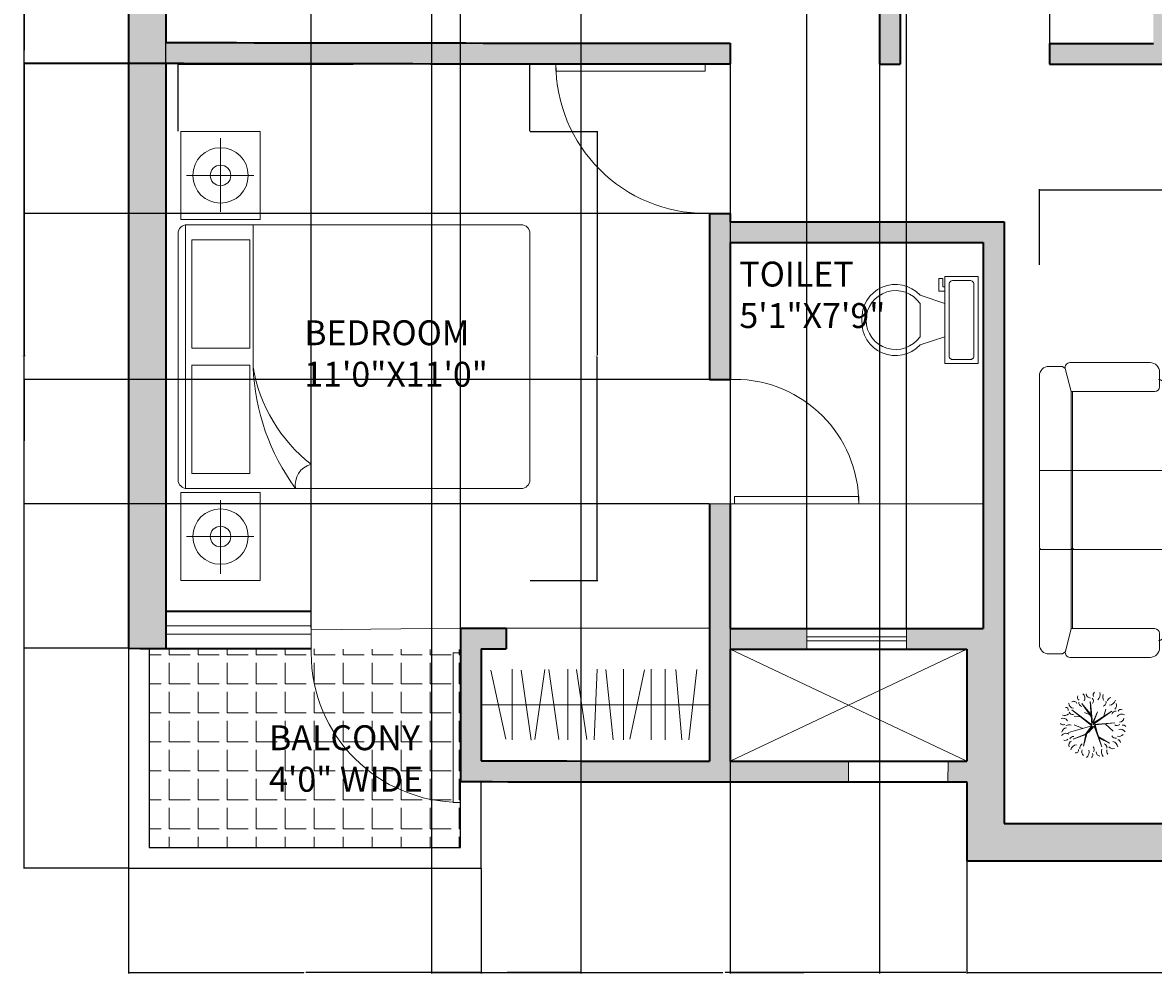
# Model space of a CAD drawing. Units: inches. Extents: x 1044 to 1567, y 918 to 1417.
# Tile 1 of 4: x 1044 to 1316, y 918 to 1148. Entities that reach past the tile are written whole.
import ezdxf

# ---------------------------------------------------------------- set-up
doc = ezdxf.new("R2010")
doc.units = ezdxf.units.IN
for name, color, linetype, lineweight in [('A-ANNO-DIMS', 2, 'Continuous', 18), ('A-AREA-IDEN', 7, 'Continuous', 18), ('A-FLOR', 7, 'Continuous', 13), ('A-FLOR-CASE', 8, 'Continuous', 18), ('A-FLOR-FIXT', 9, 'Continuous', 18), ('A-FLOR-OPEN', 8, 'Continuous', 13), ('A-FLOR-PATT', 9, 'Continuous', 13), ('A-FURN', 8, 'Continuous', 18), ('A-GLAZ', 4, 'Continuous', 13), ('A-WALL', 7, 'Continuous', 35), ('A-WALL-PATT', 252, 'Continuous', 13), ('A-WALL-PRPT', 7, 'Continuous', 25), ('door', 4, 'Continuous', 18)]:
    doc.layers.add(name, color=color, linetype=linetype, lineweight=lineweight)
doc.styles.get("Standard").update_dxf_attribs({"font": 'arial.ttf'})
doc.dimstyles.get("Standard").update_dxf_attribs({"dimtxt": 0.18, "dimasz": 0.18, "dimexe": 0.18, "dimexo": 0.0625, "dimgap": 0.09, "dimtad": 0, "dimtih": 1, "dimtoh": 1, "dimdec": 4, "dimzin": 0, "dimdsep": 46, "dimtxsty": 'Standard', "dimcen": 0.09, "dimadec": 0, "dimazin": 0, "dimtfac": 1, "dimtdec": 4, "dimtofl": 0, "dimtmove": 0, "dimatfit": 3, "dimfxl": 1, "dimtolj": 1, "dimtzin": 0, "dimarcsym": 0})

# ---------------------------------------------------------------- blocks, each defined once
blk = doc.blocks.new('*U4')
for p, q in [((0, 0), (0, 6)), ((36, 0), (36, 6))]:
    blk.add_line(p, q)
blk.add_lwpolyline([(0, 0), (0, -36), (1.75, -36), (1.75, 0)], close=True)
blk.add_arc((0, 0), 36, 270, 0)
blk = doc.blocks.new('*U3')
for p, q in [((-30, 0), (-30, -6)), ((0, 0), (0, -6))]:
    blk.add_line(p, q)
blk.add_lwpolyline([(0, 0), (0, 30), (-1.75, 30), (-1.75, 0)], close=True)
blk.add_arc((0, 0), 30, 90, 180)
blk = doc.blocks.new('*U12')
for p, q in [((-36, 0), (-36, 6)), ((0, 0), (0, 6))]:
    blk.add_line(p, q)
blk.add_lwpolyline([(0, 0), (0, -36), (-1.75, -36), (-1.75, 0)], close=True)
blk.add_arc((0, 0), 36, 180, 270)
blk = doc.blocks.new('A$C151D5484')
for p, q in [((1369.5, 1892.5), (769.5, 1892.5)), ((1369, 1877.5), (1369, 1123.6)), ((1369.5, 1108.6), (1369.5, 1892.5)), ((2468.2, 1892.5), (1384, 1892.5)), ((1869.5, 1108.6), (1869.5, 1892.5)), ((709.5, 1762.5), (709.5, 1832.5)), ((2528.2, 1756), (2528.2, 1832.5)), ((709.5, 1756), (709.5, 1762.5)), ((725.3, 1728.6), (869.5, 1692.5)), ((2514.2, 1729), (2368.2, 1692.5)), ((202.4, 1601.7), (169.9, 1679.1)), ((169.9, 1679.1), (199.5, 1598.8)), ((254.6, 1562.3), (213.8, 1708.1)), ((213.8, 1708.1), (254.6, 1560.8)), ((237.9, 1617.5), (261.5, 1673.1)), ((356.6, 1687.9), (254.6, 1562.3)), ((261.5, 1560.8), (356.6, 1687.9)), ((312.8, 1632.7), (315.2, 1673.1)), ((688, 1193.1), (688, 1699.5)), ((869.5, 1163.1), (869.5, 1692.5)), ((1369.5, 1692.5), (869.5, 1692.5)), ((1369.5, 1684.5), (869.5, 1684.5)), ((2368.2, 1692.5), (1384, 1692.5)), ((2368.2, 1684.5), (1384, 1684.5)), ((2368.2, 1163.1), (2368.2, 1692.5)), ((2551.5, 1193.1), (2551.5, 1699.9)), ((199.5, 1598.8), (126.1, 1614.5)), ((126.1, 1614.5), (203.9, 1591.9)), ((254.6, 1560.8), (202.4, 1601.7)), ((203.9, 1591.9), (253.2, 1557.9)), ((253.2, 1557.9), (212.3, 1582.5)), ((212.3, 1582.5), (253.2, 1546.1)), ((316.7, 1566.8), (396, 1625.4)), ((396, 1625.4), (321.1, 1560.8)), ((321.1, 1560.8), (340.3, 1608.6)), ((253.2, 1546.1), (123.1, 1497.8)), ((123.1, 1497.8), (260.1, 1544.6)), ((144.8, 1448.6), (187.2, 1521.4)), ((177.3, 1514.1), (144.8, 1448.6)), ((260.1, 1544.6), (177.3, 1514.1)), ((187.2, 1521.4), (261.5, 1540.2)), ((409.3, 1572.7), (261.5, 1560.8)), ((261.5, 1540.2), (273.4, 1416.5)), ((273.4, 1416.5), (264.5, 1553.5)), ((264.5, 1553.5), (347.2, 1433.8)), ((271.9, 1556.4), (403.4, 1569.7)), ((343.3, 1524.4), (271.9, 1556.4)), ((271.9, 1552), (343.3, 1524.4)), ((347.2, 1433.8), (271.9, 1552)), ((403.4, 1569.7), (316.7, 1566.8)), ((267.9, 1476.6), (221.2, 1427.3)), ((317.2, 1485.5), (360, 1472.6)), ((699.4, 1077.4), (192.6, 1077.4)), ((748, 1133.1), (839.5, 1133.1)), ((1369.5, 1108.6), (823.9, 1108.6)), ((2415.6, 1108.6), (1384, 1108.6)), ((2491.5, 1133.1), (2398.2, 1133.1)), ((136.6, 1054.2), (60, 1054.2)), ((163.5, 1040.2), (200, 894.2)), ((759.4, 1017.4), (759.4, 924.2)), ((0, 994.2), (0, 338.9)), ((783.9, 941.5), (783.9, 393.4)), ((2408.8, 932.3), (2408.8, 839.1)), ((2468.8, 992.3), (2975.6, 992.3)), ((3004.7, 955.1), (2968.2, 809.1)), ((3031.7, 969.1), (3108.2, 969.1)), ((729.4, 894.2), (200, 894.2)), ((200, 894.2), (200, 438.9)), ((208, 894.2), (208, 438.9)), ((1932.2, 900), (1132.2, 900)), ((3168.2, 909.1), (3168.2, 253.8)), ((1082.2, 50), (1082.2, 850)), ((1182.2, 100), (1182.2, 800)), ((1882.2, 800), (1182.2, 800)), ((1882.2, 100), (1882.2, 800)), ((1982.2, 50), (1982.2, 850)), ((2384.3, 856.4), (2384.3, 308.3)), ((2438.8, 809.1), (2968.2, 809.1)), ((2960.2, 809.1), (2960.2, 353.8)), ((2968.2, 809.1), (2968.2, 353.8)), ((1882.2, 647.3), (1183.2, 237)), ((1882.2, 695.3), (1190.6, 289.3)), ((164, 294.7), (200, 438.9)), ((729.4, 438.9), (200, 438.9)), ((759.4, 317.5), (759.4, 408.9)), ((2408.8, 232.4), (2408.8, 323.8)), ((2438.8, 353.8), (2968.2, 353.8)), ((3004.3, 209.6), (2968.2, 353.8)), ((130, 278.9), (60, 278.9)), ((136.6, 278.9), (130, 278.9)), ((699.4, 257.5), (193.1, 257.5)), ((2468.8, 172.4), (2975.2, 172.4)), ((3031.7, 193.8), (3038.2, 193.8)), ((3038.2, 193.8), (3108.2, 193.8)), ((1882.2, 100), (1182.2, 100)), ((1932.2, 0), (1132.2, 0))]:
    blk.add_line(p, q)
for centre, radius, start, end in [((769.5, 1832.5), 60, 90, 180), ((1384, 1877.5), 15, 90, 180), ((2468.2, 1832.5), 60, 0, 90), ((187.1, 1731), 24.5, 161.81925, 230.08176), ((177.5, 1725), 30.6, 324.97446, 61.37923), ((205.1, 1714.3), 38.8, 10.87616, 75.44791), ((232.7, 1706.8), 29.4, 330.50948, 39.29199), ((288.1, 1741.4), 26.5, 134.25765, 198.59266), ((270.3, 1743.8), 33.6, 300.94824, 20.57839), ((354.9, 1734.8), 35.6, 159.72014, 225.64891), ((356.2, 1726.1), 15.5, 253.49335, 4.46973), ((718, 1699.5), 30, 75.96376, 180), ((739.5, 1756), 30, 180, 255.96376), ((2498.2, 1756), 30, 284.03624, 0), ((2521.5, 1699.9), 30, 0, 104.03624), ((101.2, 1661.9), 17.2, 166.54191, 283.47743), ((97.2, 1657.3), 37.3, 1.63276, 82.02679), ((134, 1678.6), 27.3, 23.47529, 113.45596), ((162.1, 1676.6), 26.2, 357.17243, 67.23647), ((352.5, 1680.1), 26.5, 112.57231, 188.33354), ((400.1, 1673.2), 34.4, 93.31893, 173.19037), ((385.7, 1677.6), 24.4, 295.45365, 26.6852), ((434, 1633.1), 18.9, 56.81507, 154.01934), ((1384, 1677.5), 15, 90, 180), ((1384, 1669.5), 15, 90, 180), ((87.4, 1616.2), 38, 212.11699, 291.72753), ((92.9, 1593.6), 31.9, 69.11699, 140.36062), ((113.9, 1603.3), 33.6, 32.88731, 96.72533), ((400.2, 1620.3), 23.4, 78.8066, 167.6391), ((430.1, 1640.4), 35.1, 239.47372, 321.75859), ((464, 1564.4), 34.3, 102.30595, 169.6849), ((71, 1577), 21.9, 219.74751, 296.0709), ((92.8, 1505.2), 29.6, 95.31956, 170.41897), ((104.7, 1572.3), 26.4, 238.78766, 311.59771), ((412, 1579.3), 27.9, 235.52479, 310.83273), ((453.3, 1557.3), 47.8, 223.81169, 284.30773), ((449.1, 1531.3), 22, 35.40933, 112.71009), ((93.9, 1448.7), 51.8, 75.20711, 128.32175), ((94.4, 1445), 22.5, 66.77542, 141.28797), ((143.4, 1427), 33.9, 128.69621, 196.24154), ((117.4, 1490.2), 24.6, 263.64998, 344.65145), ((204.2, 1410.8), 27.1, 118.80717, 193.91988), ((320.2, 1409.1), 27.9, 356.02822, 71.36976), ((403.5, 1495.1), 24.1, 193.89139, 288.90395), ((433.5, 1458.5), 49.5, 190.3005, 250.44765), ((406.6, 1435.2), 28.2, 14.10036, 78.46502), ((440.2, 1444.2), 48, 73.46423, 122.79056), ((116.6, 1437.1), 40.7, 276.54869, 346.89113), ((149.8, 1398.4), 17.7, 269.25572, 357.62866), ((220.2, 1388.5), 31.6, 161.37117, 231.75354), ((200, 1381.3), 34.2, 299.1952, 16.7189), ((240.9, 1363.2), 18.8, 298.19814, 22.19179), ((284.5, 1402.5), 27.3, 148.87476, 221.21352), ((306.7, 1385.5), 27.7, 180.25287, 263.52208), ((290.4, 1371.7), 38.6, 334.73526, 50.57812), ((340.3, 1378.7), 18.7, 329.98145, 65.66759), ((383.9, 1431.1), 26.9, 212.58173, 297.17999), ((748, 1193.1), 60, 180, 270), ((839.5, 1163.1), 30, 270, 0), ((2398.2, 1163.1), 30, 180, 270), ((2491.5, 1193.1), 60, 270, 0), ((192.6, 1047.4), 30, 90, 194.03624), ((699.4, 1017.4), 60, 0, 90), ((823.9, 1138.6), 30, 180, 270), ((2415.6, 1138.6), 30, 270, 0), ((60, 994.2), 60, 90, 180), ((136.6, 1024.2), 30, 14.03624, 90), ((753.9, 941.5), 30, 0, 90), ((2468.8, 932.3), 60, 90, 180), ((2975.6, 962.3), 30, 345.96376, 90), ((3031.7, 939.1), 30, 90, 165.96376), ((3108.2, 909.1), 60, 0, 90), ((729.4, 924.2), 30, 270, 0), ((1132.2, 850), 50, 90, 180), ((1932.2, 850), 50, 0, 90), ((2414.3, 856.4), 30, 90, 180), ((2438.8, 839.1), 30, 180, 270), ((729.4, 408.9), 30, 0, 90), ((753.9, 393.4), 30, 270, 0), ((60, 338.9), 60, 180, 270), ((136.6, 308.9), 30, 270, 345.96376), ((193.1, 287.5), 30, 165.96376, 270), ((699.4, 317.5), 60, 270, 0), ((2414.3, 308.3), 30, 180, 270), ((2438.8, 323.8), 30, 90, 180), ((2468.8, 232.4), 60, 180, 270), ((3031.7, 223.8), 30, 194.03624, 270), ((3108.2, 253.8), 60, 270, 0), ((2975.2, 202.4), 30, 270, 14.03624), ((1132.2, 50), 50, 180, 270), ((1932.2, 50), 50, 270, 0)]:
    blk.add_arc(centre, radius, start, end)
blk = doc.blocks.new('A$C3C75334F')
for p, q in [((1.9728, 2), (0.5728, 2)), ((0, 1.534), (0, 1.984)), ((0, 1.984), (0.5, 1.984)), ((0.25, 1.9525), (0.25, 1.57)), ((0.5, 1.984), (0.5, 1.534)), ((2.0228, 1.958), (0.5228, 1.958)), ((0.5228, 1.95), (0.5228, 0.05)), ((2.0228, 0.05), (2.0228, 1.95)), ((2.0529, 1.984), (2.0529, 1.534)), ((2.5529, 1.984), (2.0529, 1.984)), ((2.3029, 1.9525), (2.3029, 1.57)), ((2.5529, 1.534), (2.5529, 1.984)), ((0.6089, 1.9225), (0.6089, 1.5925)), ((1.2239, 1.9225), (0.6089, 1.9225)), ((1.2239, 1.5925), (1.2239, 1.9225)), ((1.3217, 1.5925), (1.3217, 1.9225)), ((1.3217, 1.9225), (1.9367, 1.9225)), ((1.9367, 1.9225), (1.9367, 1.5925)), ((0.457, 1.759), (0.0385, 1.759)), ((2.0959, 1.759), (2.5144, 1.759)), ((0.6089, 1.5925), (1.2239, 1.5925)), ((1.2128, 1.5739), (2.0228, 1.5739)), ((1.9367, 1.5925), (1.3217, 1.5925)), ((0.5, 1.534), (0, 1.534)), ((2.0529, 1.534), (2.5529, 1.534)), ((0.5728, 0), (1.9728, 0))]:
    blk.add_line(p, q)
for centre, radius in [((0.25, 1.759), 0.1575), ((2.3029, 1.759), 0.1575), ((0.25, 1.759), 0.0585), ((2.3029, 1.759), 0.0585)]:
    blk.add_circle(centre, radius)
for centre, radius, start, end in [((0.5728, 1.95), 0.05, 90, 180), ((1.9728, 1.95), 0.05, 0, 90), ((1.2652, 0.3179), 1.2571, 92.38351, 126.19807), ((1.3644, 0.6928), 0.894, 99.75657, 141.93721), ((0.544, 1.2137), 0.1205, 14.54629, 100.1199), ((0.5728, 0.05), 0.05, 180, 270), ((1.9728, 0.05), 0.05, 270, 0)]:
    blk.add_arc(centre, radius, start, end)
blk = doc.blocks.new('*U14')
for p, q in [((9.5, -6), (9.5, -2)), ((-8, -8.5), (-8, -8)), ((-7, -8), (-7, -9.5)), ((-4, -8), (-6, -14)), ((4, -8), (6, -14)), ((-10, -8.5), (-8, -8.5)), ((-10, -9.5), (-10, -8.5)), ((-7, -9.5), (-10, -9.5)), ((4, -14), (-4, -14))]:
    blk.add_line(p, q)
blk.add_lwpolyline([(10.5, -8), (10.5, 0), (-10.5, 0), (-10.5, -8)], close=True)
for points in [[(-9.5, -2), (-9.5, -6)], [(8.5, -1), (-8.5, -1)], [(-8.5, -7), (8.5, -7)]]:
    blk.add_lwpolyline(points)
for centre, radius, start, end in [((-8.625, -1.875), 0.8839, 81.8699, 188.1301), ((8.625, -1.875), 0.8839, 351.8699, 98.1301), ((-8.625, -6.125), 0.8839, 171.869898, 278.1301), ((8.625, -6.125), 0.8839, 261.8699, 8.1301), ((-0.4772, -19.9188), 8.0953, 133.01722, 273.38), ((0.0374, -19.8731), 7.127, 124.50543, 269.7), ((-0.0373, -19.8731), 7.127, 270.3, 55.4946), ((0.4773, -19.9188), 8.0953, 266.62, 46.9828)]:
    blk.add_arc(centre, radius, start, end)
blk = doc.blocks.new('*D18')
at = {"layer": 'A-ANNO-DIMS', "color": 0, "lineweight": -2, "transparency": 16777216}
for p, q in [((1165.96, 1121.32), (1182.31, 1121.32)), ((1182.13, 1121.14), (1182.13, 1067.4)), ((1182.13, 1013.29), (1182.13, 1067.03)), ((1165.96, 1013.11), (1182.31, 1013.11))]:
    blk.add_line(p, q, dxfattribs=at)
at = {"layer": 'A-ANNO-DIMS', "color": 0, "transparency": 16777216}
for points in [[(1182.1, 1121.14), (1182.16, 1121.14), (1182.13, 1121.32)], [(1182.1, 1013.29), (1182.16, 1013.29), (1182.13, 1013.11)]]:
    blk.add_solid(points, dxfattribs=at)
at = {"layer": 'Defpoints', "color": 0, "transparency": 16777216}
for p in [(1165.9, 1121.32), (1182.13, 1121.32), (1165.9, 1013.11)]:
    blk.add_point(p, dxfattribs=at)
at = {"layer": 'A-ANNO-DIMS', "color": 0, "transparency": 16777216, "insert": (1182.13, 1067.22), "char_height": 0.18, "attachment_point": 5}
blk.add_mtext('\\A1;BED GROUP 108', dxfattribs=at)
blk = doc.blocks.new('*D19')
at = {"layer": 'A-ANNO-DIMS', "color": 0, "lineweight": -2, "transparency": 16777216}
for p, q in [((1081.12, 1121.39), (1081.12, 1137.73)), ((1081.3, 1137.55), (1123.29, 1137.55)), ((1165.72, 1137.55), (1123.73, 1137.55)), ((1165.9, 1121.39), (1165.9, 1137.73))]:
    blk.add_line(p, q, dxfattribs=at)
at = {"layer": 'A-ANNO-DIMS', "color": 0, "transparency": 16777216}
for points in [[(1081.3, 1137.58), (1081.3, 1137.52), (1081.12, 1137.55)], [(1165.72, 1137.58), (1165.72, 1137.52), (1165.9, 1137.55)]]:
    blk.add_solid(points, dxfattribs=at)
at = {"layer": 'Defpoints', "color": 0, "transparency": 16777216}
for p in [(1081.12, 1137.55), (1081.12, 1121.32), (1165.9, 1121.32)]:
    blk.add_point(p, dxfattribs=at)
at = {"layer": 'A-ANNO-DIMS', "color": 0, "transparency": 16777216, "insert": (1123.51, 1137.55), "char_height": 0.18, "attachment_point": 5}
blk.add_mtext('\\A1;85', dxfattribs=at)
blk = doc.blocks.new('*D23')
at = {"layer": 'A-ANNO-DIMS', "color": 0, "lineweight": -2, "transparency": 16777216}
for p, q in [((1288.72, 1089.17), (1288.72, 1107.4)), ((1288.9, 1107.22), (1324.56, 1107.22)), ((1360.66, 1107.22), (1325, 1107.22)), ((1360.84, 1089.17), (1360.84, 1107.4))]:
    blk.add_line(p, q, dxfattribs=at)
at = {"layer": 'A-ANNO-DIMS', "color": 0, "transparency": 16777216}
for points in [[(1288.9, 1107.25), (1288.9, 1107.19), (1288.72, 1107.22)], [(1360.66, 1107.25), (1360.66, 1107.19), (1360.84, 1107.22)]]:
    blk.add_solid(points, dxfattribs=at)
at = {"layer": 'Defpoints', "color": 0, "transparency": 16777216}
for p in [(1288.72, 1107.22), (1288.72, 1089.11), (1360.84, 1089.11)]:
    blk.add_point(p, dxfattribs=at)
at = {"layer": 'A-ANNO-DIMS', "color": 0, "transparency": 16777216, "insert": (1324.78, 1107.22), "char_height": 0.18, "attachment_point": 5}
blk.add_mtext('\\A1;72', dxfattribs=at)
blk = doc.blocks.new('*D31')
at = {"layer": 'A-ANNO-DIMS', "color": 0, "lineweight": -2, "transparency": 16777216}
for p, q in [((1087.11, 1337.65), (1043.83, 1337.65)), ((1044.01, 1337.47), (1044.01, 1140.89)), ((1044.01, 943.95), (1044.01, 1140.53)), ((1069.11, 943.77), (1043.83, 943.77))]:
    blk.add_line(p, q, dxfattribs=at)
at = {"layer": 'A-ANNO-DIMS', "color": 0, "transparency": 16777216}
for points in [[(1043.98, 1337.47), (1044.04, 1337.47), (1044.01, 1337.65)], [(1043.98, 943.95), (1044.04, 943.95), (1044.01, 943.77)]]:
    blk.add_solid(points, dxfattribs=at)
at = {"layer": 'Defpoints', "color": 0, "transparency": 16777216}
for p in [(1044.01, 1337.65), (1087.18, 1337.65), (1069.18, 943.77)]:
    blk.add_point(p, dxfattribs=at)
at = {"layer": 'A-ANNO-DIMS', "color": 0, "transparency": 16777216, "insert": (1044.01, 1140.71), "char_height": 0.18, "attachment_point": 5}
blk.add_mtext('\\A1;393.9', dxfattribs=at)
blk = doc.blocks.new('*D32')
at = {"layer": 'A-ANNO-DIMS', "color": 0, "lineweight": -2, "transparency": 16777216}
for p, q in [((1069.18, 943.7), (1069.18, 918.44)), ((1154.17, 943.7), (1154.17, 918.44)), ((1069.36, 918.62), (1111.45, 918.62)), ((1153.99, 918.62), (1111.89, 918.62))]:
    blk.add_line(p, q, dxfattribs=at)
at = {"layer": 'A-ANNO-DIMS', "color": 0, "transparency": 16777216}
for points in [[(1069.36, 918.65), (1069.36, 918.59), (1069.18, 918.62)], [(1153.99, 918.65), (1153.99, 918.59), (1154.17, 918.62)]]:
    blk.add_solid(points, dxfattribs=at)
at = {"layer": 'Defpoints', "color": 0, "transparency": 16777216}
for p in [(1069.18, 943.77), (1154.17, 943.77), (1154.17, 918.62)]:
    blk.add_point(p, dxfattribs=at)
at = {"layer": 'A-ANNO-DIMS', "color": 0, "transparency": 16777216, "insert": (1111.67, 918.62), "char_height": 0.18, "attachment_point": 5}
blk.add_mtext('\\A1;85', dxfattribs=at)
blk = doc.blocks.new('*D33')
at = {"layer": 'A-ANNO-DIMS', "color": 0, "lineweight": -2, "transparency": 16777216}
for p, q in [((1154.17, 943.7), (1154.17, 918.44)), ((1271.18, 945.49), (1271.18, 918.44)), ((1154.35, 918.62), (1212.39, 918.62)), ((1271, 918.62), (1212.95, 918.62))]:
    blk.add_line(p, q, dxfattribs=at)
at = {"layer": 'A-ANNO-DIMS', "color": 0, "transparency": 16777216}
for points in [[(1154.35, 918.65), (1154.35, 918.59), (1154.17, 918.62)], [(1271, 918.65), (1271, 918.59), (1271.18, 918.62)]]:
    blk.add_solid(points, dxfattribs=at)
at = {"layer": 'Defpoints', "color": 0, "transparency": 16777216}
for p in [(1154.17, 943.77), (1271.18, 945.56), (1271.18, 918.62)]:
    blk.add_point(p, dxfattribs=at)
at = {"layer": 'A-ANNO-DIMS', "color": 0, "transparency": 16777216, "insert": (1212.67, 918.62), "char_height": 0.18, "attachment_point": 5}
blk.add_mtext('\\A1;117', dxfattribs=at)
blk = doc.blocks.new('*D34')
at = {"layer": 'A-ANNO-DIMS', "color": 0, "lineweight": -2, "transparency": 16777216}
for p, q in [((1271.18, 945.49), (1271.18, 918.44)), ((1452.18, 945.57), (1452.18, 918.44)), ((1271.36, 918.62), (1361.41, 918.62)), ((1452, 918.62), (1361.94, 918.62))]:
    blk.add_line(p, q, dxfattribs=at)
at = {"layer": 'A-ANNO-DIMS', "color": 0, "transparency": 16777216}
for points in [[(1271.36, 918.65), (1271.36, 918.59), (1271.18, 918.62)], [(1452, 918.65), (1452, 918.59), (1452.18, 918.62)]]:
    blk.add_solid(points, dxfattribs=at)
at = {"layer": 'Defpoints', "color": 0, "transparency": 16777216}
for p in [(1271.18, 945.56), (1452.18, 945.63), (1452.18, 918.62)]:
    blk.add_point(p, dxfattribs=at)
at = {"layer": 'A-ANNO-DIMS', "color": 0, "transparency": 16777216, "insert": (1361.68, 918.62), "char_height": 0.18, "attachment_point": 5}
blk.add_mtext('\\A1;181', dxfattribs=at)
blk = doc.blocks.new('*D46')
at = {"layer": 'A-ANNO-DIMS', "color": 0, "lineweight": -2, "transparency": 16777216}
for p, q in [((1078.11, 1137.75), (1043.83, 1137.75)), ((1044.01, 1137.57), (1044.01, 1067.44)), ((1044.01, 996.95), (1044.01, 1067.08)), ((1069.11, 996.77), (1043.83, 996.77))]:
    blk.add_line(p, q, dxfattribs=at)
at = {"layer": 'A-ANNO-DIMS', "color": 0, "transparency": 16777216}
for points in [[(1043.98, 1137.57), (1044.04, 1137.57), (1044.01, 1137.75)], [(1043.98, 996.95), (1044.04, 996.95), (1044.01, 996.77)]]:
    blk.add_solid(points, dxfattribs=at)
at = {"layer": 'Defpoints', "color": 0, "transparency": 16777216}
for p in [(1044.01, 1137.75), (1078.18, 1137.75), (1069.18, 996.77)]:
    blk.add_point(p, dxfattribs=at)
at = {"layer": 'A-ANNO-DIMS', "color": 0, "transparency": 16777216, "insert": (1044.01, 1067.26), "char_height": 0.18, "attachment_point": 5}
blk.add_mtext('\\A1;140.98', dxfattribs=at)
blk = doc.blocks.new('*D47')
at = {"layer": 'A-ANNO-DIMS', "color": 0, "lineweight": -2, "transparency": 16777216}
for p, q in [((1069.11, 1283.77), (1043.83, 1283.77)), ((1044.01, 1283.59), (1044.01, 1210.94)), ((1044.01, 1137.93), (1044.01, 1210.58)), ((1078.11, 1137.75), (1043.83, 1137.75))]:
    blk.add_line(p, q, dxfattribs=at)
at = {"layer": 'A-ANNO-DIMS', "color": 0, "transparency": 16777216}
for points in [[(1043.98, 1283.59), (1044.04, 1283.59), (1044.01, 1283.77)], [(1043.98, 1137.93), (1044.04, 1137.93), (1044.01, 1137.75)]]:
    blk.add_solid(points, dxfattribs=at)
at = {"layer": 'Defpoints', "color": 0, "transparency": 16777216}
for p in [(1044.01, 1283.77), (1069.18, 1283.77), (1078.18, 1137.75)]:
    blk.add_point(p, dxfattribs=at)
at = {"layer": 'A-ANNO-DIMS', "color": 0, "transparency": 16777216, "insert": (1044.01, 1210.76), "char_height": 0.18, "attachment_point": 5}
blk.add_mtext('\\A1;146.02', dxfattribs=at)
blk = doc.blocks.new('*D48')
at = {"layer": 'A-ANNO-DIMS', "color": 0, "lineweight": -2, "transparency": 16777216}
for p, q in [((1142.18, 1274.59), (1142.18, 918.44)), ((1178.18, 1274.55), (1178.18, 918.44)), ((1142.36, 918.62), (1159.96, 918.62)), ((1178, 918.62), (1160.4, 918.62))]:
    blk.add_line(p, q, dxfattribs=at)
at = {"layer": 'A-ANNO-DIMS', "color": 0, "transparency": 16777216}
for points in [[(1142.36, 918.65), (1142.36, 918.59), (1142.18, 918.62)], [(1178, 918.65), (1178, 918.59), (1178.18, 918.62)]]:
    blk.add_solid(points, dxfattribs=at)
at = {"layer": 'Defpoints', "color": 0, "transparency": 16777216}
for p in [(1142.18, 1274.65), (1178.18, 1274.61), (1178.18, 918.62)]:
    blk.add_point(p, dxfattribs=at)
at = {"layer": 'A-ANNO-DIMS', "color": 0, "transparency": 16777216, "insert": (1160.18, 918.62), "char_height": 0.18, "attachment_point": 5}
blk.add_mtext('\\A1;36', dxfattribs=at)
blk = doc.blocks.new('*D49')
at = {"layer": 'A-ANNO-DIMS', "color": 0, "lineweight": -2, "transparency": 16777216}
for p, q in [((1078.18, 1002.26), (1078.18, 1376.67)), ((1078.36, 1376.49), (1095.46, 1376.49)), ((1113, 1376.49), (1095.9, 1376.49)), ((1113.18, 1001.71), (1113.18, 1376.67))]:
    blk.add_line(p, q, dxfattribs=at)
at = {"layer": 'A-ANNO-DIMS', "color": 0, "transparency": 16777216}
for points in [[(1078.36, 1376.52), (1078.36, 1376.46), (1078.18, 1376.49)], [(1113, 1376.52), (1113, 1376.46), (1113.18, 1376.49)]]:
    blk.add_solid(points, dxfattribs=at)
at = {"layer": 'Defpoints', "color": 0, "transparency": 16777216}
for p in [(1113.18, 1376.49), (1078.18, 1002.19), (1113.18, 1001.65)]:
    blk.add_point(p, dxfattribs=at)
at = {"layer": 'A-ANNO-DIMS', "color": 0, "transparency": 16777216, "insert": (1095.68, 1376.49), "char_height": 0.18, "attachment_point": 5}
blk.add_mtext('\\A1;35', dxfattribs=at)
blk = doc.blocks.new('*D50')
at = {"layer": 'A-ANNO-DIMS', "color": 0, "lineweight": -2, "transparency": 16777216}
for p, q in [((1113.18, 1001.71), (1113.18, 1376.67)), ((1113.36, 1376.49), (1130.96, 1376.49)), ((1149, 1376.49), (1131.4, 1376.49)), ((1149.18, 1001.71), (1149.18, 1376.67))]:
    blk.add_line(p, q, dxfattribs=at)
at = {"layer": 'A-ANNO-DIMS', "color": 0, "transparency": 16777216}
for points in [[(1113.36, 1376.52), (1113.36, 1376.46), (1113.18, 1376.49)], [(1149, 1376.52), (1149, 1376.46), (1149.18, 1376.49)]]:
    blk.add_solid(points, dxfattribs=at)
at = {"layer": 'Defpoints', "color": 0, "transparency": 16777216}
for p in [(1149.18, 1376.49), (1113.18, 1001.65), (1149.18, 1001.65)]:
    blk.add_point(p, dxfattribs=at)
at = {"layer": 'A-ANNO-DIMS', "color": 0, "transparency": 16777216, "insert": (1131.18, 1376.49), "char_height": 0.18, "attachment_point": 5}
blk.add_mtext('\\A1;36', dxfattribs=at)
blk = doc.blocks.new('*D54')
at = {"layer": 'A-ANNO-DIMS', "color": 0, "lineweight": -2, "transparency": 16777216}
for p, q in [((1209.11, 1061.59), (1043.83, 1061.59)), ((1044.01, 1061.41), (1044.01, 1046.77)), ((1044.01, 1031.77), (1044.01, 1046.41)), ((1209.11, 1031.59), (1043.83, 1031.59))]:
    blk.add_line(p, q, dxfattribs=at)
at = {"layer": 'A-ANNO-DIMS', "color": 0, "transparency": 16777216}
for points in [[(1043.98, 1061.41), (1044.04, 1061.41), (1044.01, 1061.59)], [(1043.98, 1031.77), (1044.04, 1031.77), (1044.01, 1031.59)]]:
    blk.add_solid(points, dxfattribs=at)
at = {"layer": 'Defpoints', "color": 0, "transparency": 16777216}
for p in [(1044.01, 1061.59), (1209.18, 1061.59), (1209.18, 1031.59)]:
    blk.add_point(p, dxfattribs=at)
at = {"layer": 'A-ANNO-DIMS', "color": 0, "transparency": 16777216, "insert": (1044.01, 1046.59), "char_height": 0.18, "attachment_point": 5}
blk.add_mtext('\\A1;30', dxfattribs=at)
blk = doc.blocks.new('*D55')
at = {"layer": 'A-ANNO-DIMS', "color": 0, "lineweight": -2, "transparency": 16777216}
for p, q in [((1209.86, 1137.59), (1043.83, 1137.59)), ((1044.01, 1137.41), (1044.01, 1119.77)), ((1044.01, 1101.77), (1044.01, 1119.41)), ((1209.11, 1101.59), (1043.83, 1101.59))]:
    blk.add_line(p, q, dxfattribs=at)
at = {"layer": 'A-ANNO-DIMS', "color": 0, "transparency": 16777216}
for points in [[(1043.98, 1137.41), (1044.04, 1137.41), (1044.01, 1137.59)], [(1043.98, 1101.77), (1044.04, 1101.77), (1044.01, 1101.59)]]:
    blk.add_solid(points, dxfattribs=at)
at = {"layer": 'Defpoints', "color": 0, "transparency": 16777216}
for p in [(1044.01, 1137.59), (1209.93, 1137.59), (1209.18, 1101.59)]:
    blk.add_point(p, dxfattribs=at)
at = {"layer": 'A-ANNO-DIMS', "color": 0, "transparency": 16777216, "insert": (1044.01, 1119.59), "char_height": 0.18, "attachment_point": 5}
blk.add_mtext('\\A1;36', dxfattribs=at)
blk = doc.blocks.new('*D56')
at = {"layer": 'A-ANNO-DIMS', "color": 0, "lineweight": -2, "transparency": 16777216}
for p, q in [((1214.18, 1137.52), (1214.18, 918.44)), ((1250.18, 1137.5), (1250.18, 918.44)), ((1214.36, 918.62), (1231.96, 918.62)), ((1250, 918.62), (1232.4, 918.62))]:
    blk.add_line(p, q, dxfattribs=at)
at = {"layer": 'A-ANNO-DIMS', "color": 0, "transparency": 16777216}
for points in [[(1214.36, 918.65), (1214.36, 918.59), (1214.18, 918.62)], [(1250, 918.65), (1250, 918.59), (1250.18, 918.62)]]:
    blk.add_solid(points, dxfattribs=at)
at = {"layer": 'Defpoints', "color": 0, "transparency": 16777216}
for p in [(1214.18, 1137.58), (1250.18, 1137.56), (1250.18, 918.62)]:
    blk.add_point(p, dxfattribs=at)
at = {"layer": 'A-ANNO-DIMS', "color": 0, "transparency": 16777216, "insert": (1232.18, 918.62), "char_height": 0.18, "attachment_point": 5}
blk.add_mtext('\\A1;36', dxfattribs=at)
blk = doc.blocks.new('*D57')
at = {"layer": 'A-ANNO-DIMS', "color": 0, "lineweight": -2, "transparency": 16777216}
for p, q in [((1255.18, 1137.62), (1255.18, 1376.67)), ((1255.36, 1376.49), (1272.96, 1376.49)), ((1291, 1376.49), (1273.4, 1376.49)), ((1291.18, 1142.61), (1291.18, 1376.67))]:
    blk.add_line(p, q, dxfattribs=at)
at = {"layer": 'A-ANNO-DIMS', "color": 0, "transparency": 16777216}
for points in [[(1255.36, 1376.52), (1255.36, 1376.46), (1255.18, 1376.49)], [(1291, 1376.52), (1291, 1376.46), (1291.18, 1376.49)]]:
    blk.add_solid(points, dxfattribs=at)
at = {"layer": 'Defpoints', "color": 0, "transparency": 16777216}
for p in [(1291.18, 1376.49), (1291.18, 1142.55), (1255.18, 1137.56)]:
    blk.add_point(p, dxfattribs=at)
at = {"layer": 'A-ANNO-DIMS', "color": 0, "transparency": 16777216, "insert": (1273.18, 1376.49), "char_height": 0.18, "attachment_point": 5}
blk.add_mtext('\\A1;36', dxfattribs=at)
blk = doc.blocks.new('*D62')
at = {"layer": 'A-ANNO-DIMS', "color": 0, "lineweight": -2, "transparency": 16777216}
for p, q in [((1232.68, 1001.63), (1232.68, 1376.67)), ((1232.86, 1376.49), (1244.46, 1376.49)), ((1256.5, 1376.49), (1244.9, 1376.49)), ((1256.68, 1001.62), (1256.68, 1376.67))]:
    blk.add_line(p, q, dxfattribs=at)
at = {"layer": 'A-ANNO-DIMS', "color": 0, "transparency": 16777216}
for points in [[(1232.86, 1376.52), (1232.86, 1376.46), (1232.68, 1376.49)], [(1256.5, 1376.52), (1256.5, 1376.46), (1256.68, 1376.49)]]:
    blk.add_solid(points, dxfattribs=at)
at = {"layer": 'Defpoints', "color": 0, "transparency": 16777216}
for p in [(1256.68, 1376.49), (1232.68, 1001.57), (1256.68, 1001.56)]:
    blk.add_point(p, dxfattribs=at)
at = {"layer": 'A-ANNO-DIMS', "color": 0, "transparency": 16777216, "insert": (1244.68, 1376.49), "char_height": 0.18, "attachment_point": 5}
blk.add_mtext('\\A1;24', dxfattribs=at)

msp = doc.modelspace()

# ---------------------------------------------------------------- hatches: boundary and pattern name
at = {"layer": 'A-FLOR-PATT'}
h = msp.add_hatch(dxfattribs=at)
h.set_pattern_fill('ANGLE', color=256)
h.set_pattern_definition([(0, (-17.679, -331.974), (0, 6.985), [5.08, -1.905]), (90, (-17.679, -331.974), (-6.985, 4e-16), [5.08, -1.905])])
edge = h.paths.add_edge_path()
edge.add_line((1149.177, 996.492), (1074.177, 996.767))
edge.add_line((1074.177, 996.767), (1074.177, 948.767))
edge.add_arc((1111.677, -5051.749), 6000.632, 89.6419368, 90.3580632, ccw=False)
edge.add_line((1149.177, 948.767), (1149.177, 996.492))
at = {"layer": 'A-WALL-PATT'}
h = msp.add_hatch(color=256, dxfattribs=at)
h.dxf.hatch_style = 1
h.paths.add_polyline_path([(1273.677, 1302.555, -0.0000455), (1250.177, 1302.563), (1178.177, 1302.563), (1178.177, 1274.614, 0.0000213), (1189.177, 1274.604), (1189.177, 1279.604, -0.0000116), (1183.177, 1279.609), (1183.177, 1297.563), (1250.177, 1297.563), (1250.177, 1250.563, 0.0000097), (1255.177, 1250.561), (1255.177, 1293.561, 0.0000358), (1273.677, 1293.555)])
h.paths.add_polyline_path([(1339.177, 1302.556, -0.0000348), (1321.176, 1302.553, -0.0000455), (1297.677, 1302.552), (1297.677, 1293.552, 0.0000358), (1316.177, 1293.552), (1316.177, 1190.552, -0.0001179), (1255.177, 1190.561), (1255.177, 1220.561, -0.0000097), (1250.177, 1220.563), (1250.177, 1137.563, 0.0000097), (1255.177, 1137.561), (1255.177, 1185.561, 0.0001179), (1316.177, 1185.552), (1316.177, 1142.552, -0.0000483), (1291.177, 1142.552), (1291.177, 1137.552, 0.000058), (1321.177, 1137.553), (1321.177, 1236.553, 0.0000348), (1339.177, 1236.556), (1339.177, 1245.556, -0.0000348), (1321.177, 1245.553), (1321.177, 1293.544), (1321.174, 1293.553, 0.0000348), (1339.177, 1293.556)])
h = msp.add_hatch(color=256, dxfattribs=at)
h.dxf.hatch_style = 1
h.paths.add_polyline_path([(1092.177, 1283.727, -0.0000445), (1069.177, 1283.767), (1069.177, 996.767, 0.0000174), (1078.177, 996.751), (1078.177, 1137.751, 0.0002628), (1214.177, 1137.584), (1214.177, 1142.584, -0.0002628), (1078.177, 1142.751), (1078.177, 1274.751, 0.0000271), (1092.177, 1274.727)])
h = msp.add_hatch(color=256, dxfattribs=at)
h.dxf.hatch_style = 1
h.paths.add_polyline_path([(1476.177, 1101.635), (1452.177, 1101.635, -0.0000174), (1443.177, 1101.625), (1443.177, 954.625, -0.0003145), (1280.177, 954.554), (1280.177, 1099.554, -0.0001275), (1214.177, 1099.584), (1214.177, 1101.584, -0.0000097), (1209.177, 1101.587), (1209.177, 1061.587, 0.0000097), (1214.177, 1061.584), (1214.177, 1094.584, 0.0001178), (1275.177, 1094.555), (1275.177, 1001.555, -0.0000357), (1256.677, 1001.561), (1256.674, 996.561, 0.000028), (1271.177, 996.556), (1271.177, 969.556, -0.0000087), (1266.677, 969.557), (1266.674, 964.557, 0.0000087), (1271.177, 964.556), (1271.177, 945.556, 0.0003493), (1452.177, 945.635), (1452.177, 1092.635), (1476.177, 1092.635)])
h = msp.add_hatch(color=256, dxfattribs=at)
h.dxf.hatch_style = 1
h.paths.add_polyline_path([(1232.677, 1001.572, -0.0000357), (1214.177, 1001.584), (1214.177, 1031.584, -0.0000097), (1209.177, 1031.587), (1209.177, 969.587, -0.0001061), (1154.177, 969.64), (1154.177, 996.64, 0.0000116), (1160.177, 996.633), (1160.177, 1001.633, -0.0000212), (1149.177, 1001.646), (1149.177, 964.645, 0.0001804), (1242.674, 964.567), (1242.677, 969.567, -0.000055), (1214.177, 969.584), (1214.177, 996.584, 0.0000357), (1232.674, 996.572)])

# ---------------------------------------------------------------- linework, layer by layer
at = {"layer": 'A-FLOR'}
msp.add_line((1149.177, 1001.646), (1113.177, 1001.194), dxfattribs=at)
msp.add_arc((1305.177, 130508.416), 129476.864, 269.95751832, 269.98672755, dxfattribs=at)
at = {"layer": 'A-FLOR-CASE'}
for p, q in [((1160.177, 1001.633), (1209.177, 1001.633)), ((1156.483, 991.54), (1160.062, 974.885)), ((1161.637, 991.732), (1161.637, 974.696)), ((1166.23, 974.638), (1163.764, 991.494)), ((1169.542, 991.646), (1167.128, 974.782)), ((1170.45, 991.643), (1172.897, 974.784)), ((1175.033, 991.732), (1175.033, 974.696)), ((1177.158, 991.644), (1179.605, 974.784)), ((1181.379, 974.703), (1182.082, 991.725)), ((1184.214, 991.688), (1185.945, 974.74)), ((1188.428, 991.732), (1188.428, 974.696)), ((1193.531, 991.549), (1190.023, 974.879)), ((1195.126, 991.732), (1195.126, 974.696)), ((1198.475, 991.732), (1198.475, 974.696)), ((1201.1, 991.701), (1202.536, 974.726)), ((1204.201, 974.752), (1206.145, 991.676)), ((1154.177, 983.14), (1209.177, 983.14))]:
    msp.add_line(p, q, dxfattribs=at)
at = {"layer": 'A-FLOR-OPEN'}
for p, q in [((1271.177, 969.556), (1214.177, 996.584)), ((1214.177, 969.584), (1271.177, 996.556))]:
    msp.add_line(p, q, dxfattribs=at)
at = {"layer": 'A-GLAZ'}
for p, q in [((1113.177, 1005.694), (1113.177, 996.694)), ((1113.177, 1002.194), (1078.177, 1002.194)), ((1232.677, 1001.571), (1232.674, 996.571)), ((1256.677, 1001.56), (1256.674, 996.56)), ((1113.177, 1000.194), (1078.177, 1000.194)), ((1256.675, 998.56), (1232.675, 998.571)), ((1256.676, 999.56), (1232.676, 999.571)), ((1242.677, 969.567), (1242.674, 964.567)), ((1266.677, 969.555), (1266.674, 964.555))]:
    msp.add_line(p, q, dxfattribs=at)
at = {"layer": 'A-WALL'}
for p, q in [((1069.177, 1283.767), (1069.177, 996.767)), ((1078.177, 1274.751), (1078.177, 1142.751)), ((1250.177, 1220.563), (1250.177, 1137.563)), ((1255.177, 1185.561), (1255.177, 1137.561)), ((1214.177, 1142.587), (1214.177, 1137.584)), ((1291.177, 1142.552), (1291.177, 1137.552)), ((1078.177, 1137.751), (1078.177, 996.751)), ((1209.177, 1101.587), (1209.177, 1061.587)), ((1214.177, 1101.584), (1214.177, 1099.584)), ((1280.177, 1099.554), (1280.177, 954.554)), ((1214.177, 1094.584), (1214.177, 1061.584)), ((1275.177, 1094.555), (1275.177, 1001.555)), ((1209.177, 1031.587), (1209.177, 969.587)), ((1214.177, 1031.584), (1214.177, 1001.584)), ((1149.177, 1001.646), (1149.177, 964.645)), ((1160.177, 1001.64), (1160.177, 996.633)), ((1154.177, 996.64), (1154.177, 969.64)), ((1214.177, 996.584), (1214.177, 969.584)), ((1271.177, 996.556), (1271.177, 969.556)), ((1271.177, 964.556), (1271.177, 945.556))]:
    msp.add_line(p, q, dxfattribs=at)
for radius, start, end in [(129365.864, 269.89946228, 269.95969635), (129365.864, 269.99379944, 270.00487187), (129370.864, 269.89946617, 269.95969791), (129370.864, 269.97564159, 269.977856), (129370.864, 269.99379968, 270.00708608), (129406.864, 269.95749534, 269.95970912), (129408.864, 269.95970974, 269.98893125), (129413.864, 269.9597113, 269.98671801), (129446.864, 269.95750847, 269.95972157), (129502.864, 269.89956864, 269.91505366), (129506.864, 269.93098324, 269.93584981), (129506.864, 269.95974023, 269.98672755), (129511.864, 269.89559403, 269.91505957), (129511.864, 269.9331979, 269.93585229), (129511.864, 269.95974179, 269.98495847), (129538.864, 269.93321182, 269.95753865), (129538.864, 269.95975018, 269.98496161), (129543.864, 269.93100296, 269.98496219), (129553.864, 269.98894364, 270.06103113), (129562.864, 269.98496439, 270.06500691)]:
    msp.add_arc((1305.177, 130508.416), radius, start, end, dxfattribs=at)
at = {"layer": 'A-WALL-PRPT'}
for p, q in [((1069.177, 996.767), (1069.177, 943.767)), ((1074.177, 996.767), (1074.177, 948.767)), ((1149.177, 948.767), (1149.196, 964.645)), ((1154.171, 943.767), (1154.196, 964.639)), ((1074.177, 948.767), (1149.177, 948.767)), ((1069.177, 943.767), (1154.171, 943.767))]:
    msp.add_line(p, q, dxfattribs=at)

# ---------------------------------------------------------------- block references
at = {"layer": 'A-FLOR-FIXT', "rotation": 270}
msp.add_blockref('*U14', (1273.927, 1075.872), dxfattribs=at)
at = {"layer": 'A-FURN', "rotation": 90}
for name, p, xscale, yscale, zscale in [('A$C3C75334F', (1165.899, 1013.109), 42.38879344284466, 42.38879344284466, 42.38879344284466), ('A$C151D5484', (1360.841, 968.371), 0.0381098975720578, 0.0381098975720578, 0.0381098975720578)]:
    msp.add_blockref(name, p, dxfattribs=dict(at, xscale=xscale, yscale=yscale, zscale=zscale))
at = {"layer": 'door', "rotation": 270}
for name, p in [('*U4', (1208.177, 1137.587)), ('*U3', (1215.177, 1031.587))]:
    msp.add_blockref(name, p, dxfattribs=at)
at = {"layer": 'door'}
msp.add_blockref('*U12', (1149.177, 995.646), dxfattribs=at)

# ---------------------------------------------------------------- texts
at = {"layer": 'A-AREA-IDEN', "char_height": 6, "attachment_point": 1}
for s, insert in [('TOILET\\P5\'1"X7\'9"', (1216.394, 1089.957)), ('BEDROOM\\P11\'0"X11\'0"', (1111.511, 1075.814)), ('BALCONY\\P4\'0" WIDE', (1103.031, 978.221))]:
    msp.add_mtext_dynamic_manual_height_columns(s, width=56.12489, gutter_width=12.5, heights=[0], dxfattribs=dict(at, insert=insert))

# ---------------------------------------------------------------- dimensions: what is measured, and where the dimension line sits
at = {"layer": 'A-ANNO-DIMS'}
for base, p1, p2, picture, middle in [((1113.177, 1376.486), (1078.177, 1002.194), (1113.177, 1001.646), '*D49', (1095.677, 1376.486)), ((1149.177, 1376.486), (1113.177, 1001.646), (1149.177, 1001.646), '*D50', (1131.177, 1376.486)), ((1256.677, 1376.486), (1232.677, 1001.571), (1256.677, 1001.56), '*D62', (1244.677, 1376.486)), ((1291.177, 1376.486), (1255.177, 1137.561), (1291.177, 1142.552), '*D57', (1273.177, 1376.486)), ((1178.177, 918.617), (1142.177, 1274.654), (1178.177, 1274.614), '*D48', (1160.177, 918.617)), ((1250.177, 918.617), (1214.177, 1137.584), (1250.177, 1137.563), '*D56', (1232.177, 918.617)), ((1154.171, 918.617), (1069.177, 943.767), (1154.171, 943.767), '*D32', (1111.674, 918.617)), ((1271.177, 918.617), (1154.171, 943.767), (1271.177, 945.556), '*D33', (1212.674, 918.617)), ((1452.177, 918.617), (1271.177, 945.556), (1452.177, 945.635), '*D34', (1361.677, 918.617))]:
    dim = msp.add_linear_dim(base=base, p1=p1, p2=p2, dimstyle='Standard', override={"dimdec": 0, "dimlfac": 1, "dimrnd": 0, "dimzin": 0, "dimdsep": 46, "dimlunit": 2}, dxfattribs=at)
    dim.commit()
    dim.dimension.update_dxf_attribs({"geometry": picture, "text_midpoint": middle})
for base, p1, p2, angle, override, picture, middle in [((1044.01, 1337.654), (1069.177, 943.767), (1087.177, 1337.654), 90, {"dimdec": 1, "dimlfac": 1, "dimrnd": 0, "dimzin": 0, "dimdsep": 46, "dimlunit": 2}, '*D31', (1044.01, 1140.71)), ((1044.01, 1283.767), (1078.177, 1137.751), (1069.177, 1283.767), 90, {"dimdec": 2, "dimlfac": 1, "dimrnd": 0, "dimzin": 0, "dimdsep": 46, "dimlunit": 2}, '*D47', (1044.01, 1210.759)), ((1044.01, 1137.751), (1069.177, 996.767), (1078.177, 1137.751), 90, {"dimdec": 2, "dimlfac": 1, "dimrnd": 0, "dimzin": 0, "dimdsep": 46, "dimlunit": 2}, '*D46', (1044.01, 1067.259)), ((1044.01, 1137.587), (1209.177, 1101.587), (1209.927, 1137.587), 90, {"dimdec": 0, "dimlfac": 1, "dimrnd": 0, "dimzin": 0, "dimdsep": 46, "dimlunit": 2}, '*D55', (1044.01, 1119.587)), ((1081.121, 1137.555), (1165.899, 1121.323), (1081.121, 1121.323), 180, {"dimdec": 0, "dimlfac": 1, "dimrnd": 0, "dimzin": 0, "dimdsep": 46, "dimlunit": 2}, '*D19', (1123.51, 1137.555)), ((1288.717, 1107.224), (1360.841, 1089.112), (1288.717, 1089.112), 180, {"dimdec": 0, "dimlfac": 1, "dimrnd": 0, "dimzin": 0, "dimdsep": 46, "dimlunit": 2}, '*D23', (1324.779, 1107.224)), ((1044.01, 1061.587), (1209.177, 1031.587), (1209.177, 1061.587), 90, {"dimdec": 0, "dimlfac": 1, "dimrnd": 0, "dimzin": 0, "dimdsep": 46, "dimlunit": 2}, '*D54', (1044.01, 1046.587))]:
    dim = msp.add_linear_dim(base=base, p1=p1, p2=p2, angle=angle, dimstyle='Standard', override=override, dxfattribs=at)
    dim.commit()
    dim.dimension.update_dxf_attribs({"geometry": picture, "text_midpoint": middle})
dim = msp.add_linear_dim(base=(1182.131, 1121.323), p1=(1165.899, 1013.109), p2=(1165.899, 1121.323), angle=90, text='BED GROUP <>', dimstyle='Standard', override={"dimdec": 0, "dimlfac": 1, "dimrnd": 0, "dimzin": 0, "dimdsep": 46, "dimlunit": 2}, dxfattribs=at)
dim.commit()
dim.dimension.update_dxf_attribs({"geometry": '*D18', "text_midpoint": (1182.131, 1067.216)})

doc.saveas('drawing.dxf')
